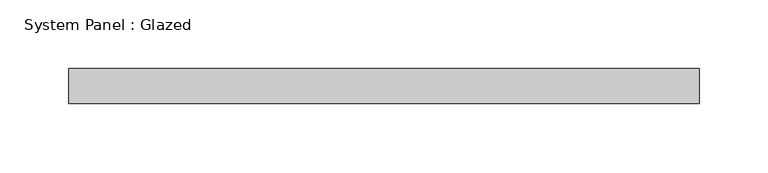
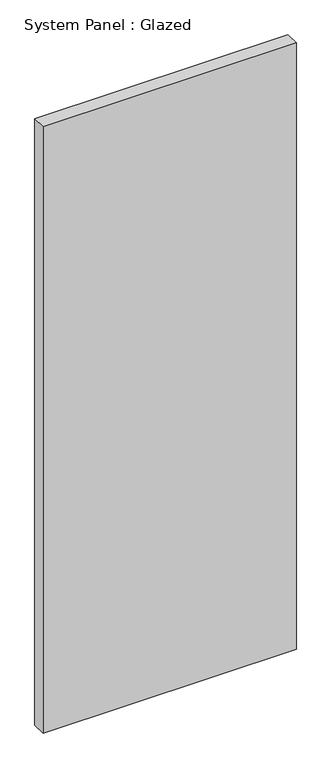
"""IFC4 building model written with IfcOpenShell, lengths in millimetres: plate geometry, System Panel : Glazed."""

from ifc_helpers import new_model, si_unit, origin, origin_with_axes, place, context, project, spatial, polyline, outline, extrude, source, transform, mapped, element, save


def system_panel_glazed_a18a7e0a(model_context):
    return source(origin(), model_context, "Body", "SweptSolid", [
        extrude(outline(polyline([(228.6, 19.05), (-228.6, 19.05), (-228.6, 44.45), (228.6, 44.45), (228.6, 19.05)])), origin_with_axes(), (0.0, 0.0, 1.0), 1155.7),
    ])


if __name__ == "__main__":
    model = new_model("IFC4")
    model_context = context("Model", 3, world=origin())
    ifc_project = project(units=[si_unit("LENGTHUNIT", "METRE", prefix="MILLI")], contexts=[model_context])
    site = spatial("IfcSite", under=ifc_project)
    building = spatial("IfcBuilding", under=site)
    placement = place(None, origin())
    system_panel_glazed_shape = system_panel_glazed_a18a7e0a(model_context)
    element("IfcPlate", 1, ObjectType="System Panel : Glazed", at=placement, inside=building, context=model_context, shape_type="MappedRepresentation", body=[
        mapped(system_panel_glazed_shape, transform((0.0, 0.0, 0.0), x_axis=(1.0, 0.0, 0.0), y_axis=(0.0, 1.0, 0.0), z_axis=(0.0, 0.0, 1.0))),
    ])
    save(model, "model.ifc")

# Revit data of these elements
# Type "System Panel : Glazed"
#   Construction Type Id = "GSP4R"
#   Analytic Construction = "1/8 in Pilkington single glazing"
#   Visual Light Transmittance = 0.9
#   Solar Heat Gain Coefficient = 0.86
#   Heat Transfer Coefficient (U) = 1.18115 BTU/(h·ft²·°F)
# Element 1 (IfcPlate, "System Panel : Glazed")
#   Materials on its faces: "Glass"
# Materials
#   "Glass": class "Glass", colour RGB 0 128 192, transparency 0.75, Description = "Soda Lime Glass", Cost = 0
